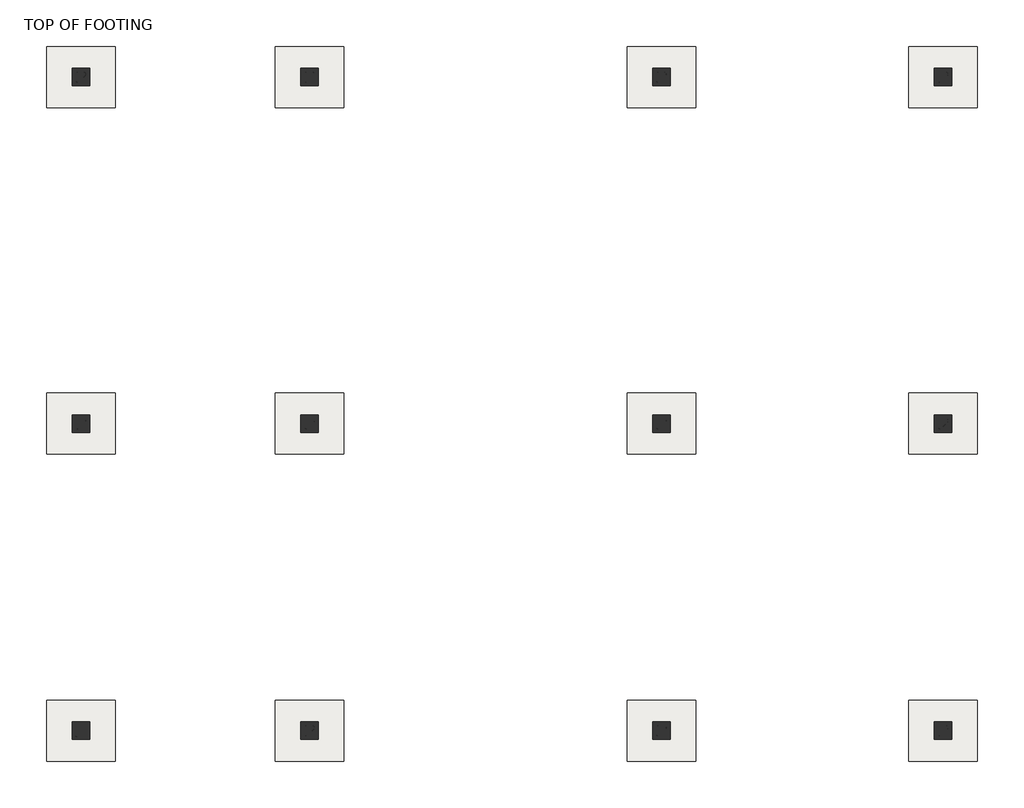
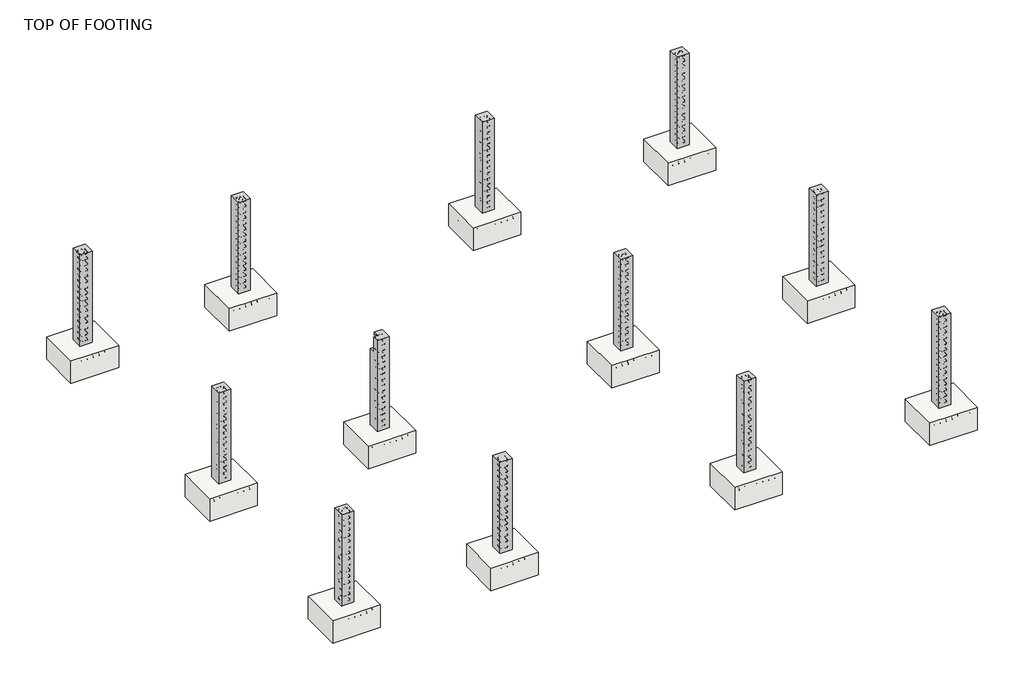
# One storey, part 1 of 6: 12 columns, 12 slabs.
"""IFC4 building model written with IfcOpenShell, lengths in millimetres."""

from ifc_helpers import new_model, si_unit, frame, origin, place, context, project, spatial, polyline, outline, extrude, faceted_brep, transform, mapped, element, save
from components import m_footing_rectangular_f0562f77

model = new_model("IFC4")

# Units and contexts
model_context = context("Model", 3, world=origin())
ifc_project = project(units=[si_unit("LENGTHUNIT", "METRE", prefix="MILLI")], contexts=[model_context])

# Site, building, storey
site = spatial("IfcSite", under=ifc_project)
building = spatial("IfcBuilding", under=site)
storey = spatial("IfcBuildingStorey", under=building, Name="TOP OF FOOTING", Elevation=-1828.8)

# Columns
placement = place(None, origin())
element("IfcColumn", 1, ObjectType="M_Concrete-Rectangular-Column : 9\" X 9\"", at=placement, inside=storey, context=model_context, shape_type="SweptSolid", body=[
    extrude(outline(polyline([(-14809.4556799, 4426.9016651), (-14809.4556799, 4198.3016651), (-15038.0556799, 4198.3016651), (-15038.0556799, 4426.9016651), (-14809.4556799, 4426.9016651)])), frame((0.0, 0.0, -1828.8), z_axis=(0.0, 0.0, 1.0), x_axis=(1.0, 0.0, 0.0)), (0.0, 0.0, 1.0), 1828.8),
])
element("IfcColumn", 2, ObjectType="M_Concrete-Rectangular-Column : 9\" X 9\"", at=placement, inside=storey, context=model_context, shape_type="Brep", body=[
    faceted_brep([(-11812.2556799, 4426.9016651, -1828.8), (-11812.2556799, 4198.3016651, -1828.8), (-12040.8556799, 4198.3016651, -1828.8), (-12040.8556799, 4426.9016651, -1828.8), (-11812.2556799, 4426.9016651, 0.0), (-11812.2556799, 4198.3016651, 0.0), (-11964.6556799, 4198.3016651, 0.0), (-12040.8556799, 4198.3016651, 0.0), (-12040.8556799, 4426.9016651, 0.0)], [[[0, 1, 2, 3]], [[4, 5, 1, 0]], [[5, 6, 7, 2, 1]], [[7, 8, 3, 2]], [[8, 4, 0, 3]], [[4, 8, 7, 6, 5]]]),
])
element("IfcColumn", 3, ObjectType="M_Concrete-Rectangular-Column : 9\" X 9\"", at=placement, inside=storey, context=model_context, shape_type="SweptSolid", body=[
    extrude(outline(polyline([(-7200.1673382, 4426.9016651), (-7200.1673382, 4198.3016651), (-7428.7673382, 4198.3016651), (-7428.7673382, 4426.9016651), (-7200.1673382, 4426.9016651)])), frame((0.0, 0.0, -1828.8), z_axis=(0.0, 0.0, 1.0), x_axis=(1.0, 0.0, 0.0)), (0.0, 0.0, 1.0), 1828.8),
])
element("IfcColumn", 4, ObjectType="M_Concrete-Rectangular-Column : 9\" X 9\"", at=placement, inside=storey, context=model_context, shape_type="SweptSolid", body=[
    extrude(outline(polyline([(-3506.4556799, 4426.9016651), (-3506.4556799, 4198.3016651), (-3735.0556799, 4198.3016651), (-3735.0556799, 4426.9016651), (-3506.4556799, 4426.9016651)])), frame((0.0, 0.0, -1828.8), z_axis=(0.0, 0.0, 1.0), x_axis=(1.0, 0.0, 0.0)), (0.0, 0.0, 1.0), 1828.8),
])
element("IfcColumn", 5, ObjectType="M_Concrete-Rectangular-Column : 9\" X 9\"", at=placement, inside=storey, context=model_context, shape_type="SweptSolid", body=[
    extrude(outline(polyline([(-3506.4556799, -118.4025279), (-3506.4556799, -347.0025279), (-3735.0556799, -347.0025279), (-3735.0556799, -118.4025279), (-3506.4556799, -118.4025279)])), frame((0.0, 0.0, -1828.8), z_axis=(0.0, 0.0, 1.0), x_axis=(1.0, 0.0, 0.0)), (0.0, 0.0, 1.0), 1828.8),
])
element("IfcColumn", 6, ObjectType="M_Concrete-Rectangular-Column : 9\" X 9\"", at=placement, inside=storey, context=model_context, shape_type="SweptSolid", body=[
    extrude(outline(polyline([(-7200.1673382, -118.4025279), (-7200.1673382, -347.0025279), (-7428.7673382, -347.0025279), (-7428.7673382, -118.4025279), (-7200.1673382, -118.4025279)])), frame((0.0, 0.0, -1828.8), z_axis=(0.0, 0.0, 1.0), x_axis=(1.0, 0.0, 0.0)), (0.0, 0.0, 1.0), 1828.8),
])
element("IfcColumn", 7, ObjectType="M_Concrete-Rectangular-Column : 9\" X 9\"", at=placement, inside=storey, context=model_context, shape_type="Brep", body=[
    faceted_brep([(-11812.2556799, -118.4025279, -1828.8), (-11812.2556799, -347.0025279, -1828.8), (-12040.8556799, -347.0025279, -1828.8), (-12040.8556799, -118.4025279, -1828.8), (-11812.2556799, -118.4025279, 0.0), (-11812.2556799, -347.0025279, 0.0), (-12040.8556799, -347.0025279, 0.0), (-12040.8556799, -232.7025279, 0.0), (-12040.8556799, -232.7025279, -300.0), (-12040.8556799, -118.4025279, -300.0), (-11964.6556799, -118.4025279, -300.0), (-11964.6556799, -118.4025279, 0.0), (-11964.6556799, -232.7025279, 0.0), (-11964.6556799, -232.7025279, -300.0)], [[[0, 1, 2, 3]], [[1, 0, 4, 5]], [[2, 1, 5, 6]], [[3, 2, 6, 7, 8, 9]], [[0, 3, 9, 10, 11, 4]], [[5, 4, 11, 12, 7, 6]], [[8, 13, 10, 9]], [[13, 12, 11, 10]], [[12, 13, 8, 7]]]),
])
element("IfcColumn", 8, ObjectType="M_Concrete-Rectangular-Column : 9\" X 9\"", at=placement, inside=storey, context=model_context, shape_type="Brep", body=[
    faceted_brep([(-14809.4556799, -118.4025279, -1828.8), (-14809.4556799, -347.0025279, -1828.8), (-15038.0556799, -347.0025279, -1828.8), (-15038.0556799, -118.4025279, -1828.8), (-14809.4556799, -118.4025279, 0.0), (-14809.4556799, -232.7025279, 0.0), (-14809.4556799, -347.0025279, 0.0), (-15038.0556799, -347.0025279, 0.0), (-15038.0556799, -118.4025279, 0.0)], [[[0, 1, 2, 3]], [[4, 5, 6, 1, 0]], [[6, 7, 2, 1]], [[7, 8, 3, 2]], [[8, 4, 0, 3]], [[4, 8, 7, 6, 5]]]),
])
element("IfcColumn", 9, ObjectType="M_Concrete-Rectangular-Column : 9\" X 9\"", at=placement, inside=storey, context=model_context, shape_type="SweptSolid", body=[
    extrude(outline(polyline([(-14809.4556799, -4145.5983349), (-14809.4556799, -4374.1983349), (-15038.0556799, -4374.1983349), (-15038.0556799, -4145.5983349), (-14809.4556799, -4145.5983349)])), frame((0.0, 0.0, -1828.8), z_axis=(0.0, 0.0, 1.0), x_axis=(1.0, 0.0, 0.0)), (0.0, 0.0, 1.0), 1828.8),
])
element("IfcColumn", 10, ObjectType="M_Concrete-Rectangular-Column : 9\" X 9\"", at=placement, inside=storey, context=model_context, shape_type="SweptSolid", body=[
    extrude(outline(polyline([(-11812.2556799, -4145.5983349), (-11812.2556799, -4374.1983349), (-12040.8556799, -4374.1983349), (-12040.8556799, -4145.5983349), (-11812.2556799, -4145.5983349)])), frame((0.0, 0.0, -1828.8), z_axis=(0.0, 0.0, 1.0), x_axis=(1.0, 0.0, 0.0)), (0.0, 0.0, 1.0), 1828.8),
])
element("IfcColumn", 11, ObjectType="M_Concrete-Rectangular-Column : 9\" X 9\"", at=placement, inside=storey, context=model_context, shape_type="SweptSolid", body=[
    extrude(outline(polyline([(-7200.1673382, -4145.5983349), (-7200.1673382, -4374.1983349), (-7428.7673382, -4374.1983349), (-7428.7673382, -4145.5983349), (-7200.1673382, -4145.5983349)])), frame((0.0, 0.0, -1828.8), z_axis=(0.0, 0.0, 1.0), x_axis=(1.0, 0.0, 0.0)), (0.0, 0.0, 1.0), 1828.8),
])
element("IfcColumn", 12, ObjectType="M_Concrete-Rectangular-Column : 9\" X 9\"", at=placement, inside=storey, context=model_context, shape_type="SweptSolid", body=[
    extrude(outline(polyline([(-3506.4556799, -4145.5983349), (-3506.4556799, -4374.1983349), (-3735.0556799, -4374.1983349), (-3735.0556799, -4145.5983349), (-3506.4556799, -4145.5983349)])), frame((0.0, 0.0, -1828.8), z_axis=(0.0, 0.0, 1.0), x_axis=(1.0, 0.0, 0.0)), (0.0, 0.0, 1.0), 1828.8),
])

# Slabs
element("IfcSlab", 13, ObjectType="M_Footing-Rectangular", at=placement, inside=storey, context=model_context, shape_type="SweptSolid", body=[
    extrude(outline(polyline([(-14473.7556799, 4712.6016651), (-14473.7556799, 3912.6016651), (-15373.7556799, 3912.6016651), (-15373.7556799, 4712.6016651), (-14473.7556799, 4712.6016651)])), frame((0.0, 0.0, -2278.8), z_axis=(0.0, 0.0, 1.0), x_axis=(1.0, 0.0, 0.0)), (0.0, 0.0, 1.0), 450.0),
])
element("IfcSlab", 14, ObjectType="M_Footing-Rectangular", at=placement, inside=storey, context=model_context, shape_type="SweptSolid", body=[
    extrude(outline(polyline([(-11476.5556799, 4712.6016651), (-11476.5556799, 3912.6016651), (-12376.5556799, 3912.6016651), (-12376.5556799, 4712.6016651), (-11476.5556799, 4712.6016651)])), frame((0.0, 0.0, -2278.8), z_axis=(0.0, 0.0, 1.0), x_axis=(1.0, 0.0, 0.0)), (0.0, 0.0, 1.0), 450.0),
])
element("IfcSlab", 15, ObjectType="M_Footing-Rectangular", at=placement, inside=storey, context=model_context, shape_type="SweptSolid", body=[
    extrude(outline(polyline([(-6864.4673382, 4712.6016651), (-6864.4673382, 3912.6016651), (-7764.4673382, 3912.6016651), (-7764.4673382, 4712.6016651), (-6864.4673382, 4712.6016651)])), frame((0.0, 0.0, -2278.8), z_axis=(0.0, 0.0, 1.0), x_axis=(1.0, 0.0, 0.0)), (0.0, 0.0, 1.0), 450.0),
])
element("IfcSlab", 16, ObjectType="M_Footing-Rectangular", at=placement, inside=storey, context=model_context, shape_type="SweptSolid", body=[
    extrude(outline(polyline([(-3170.7556799, 4712.6016651), (-3170.7556799, 3912.6016651), (-4070.7556799, 3912.6016651), (-4070.7556799, 4712.6016651), (-3170.7556799, 4712.6016651)])), frame((0.0, 0.0, -2278.8), z_axis=(0.0, 0.0, 1.0), x_axis=(1.0, 0.0, 0.0)), (0.0, 0.0, 1.0), 450.0),
])
element("IfcSlab", 17, ObjectType="M_Footing-Rectangular", at=placement, inside=storey, context=model_context, shape_type="SweptSolid", body=[
    extrude(outline(polyline([(-6864.4673382, 167.2974721), (-6864.4673382, -632.7025279), (-7764.4673382, -632.7025279), (-7764.4673382, 167.2974721), (-6864.4673382, 167.2974721)])), frame((0.0, 0.0, -2278.8), z_axis=(0.0, 0.0, 1.0), x_axis=(1.0, 0.0, 0.0)), (0.0, 0.0, 1.0), 450.0),
])
element("IfcSlab", 18, ObjectType="M_Footing-Rectangular", at=placement, inside=storey, context=model_context, shape_type="SweptSolid", body=[
    extrude(outline(polyline([(-3170.7556799, 167.2974721), (-3170.7556799, -632.7025279), (-4070.7556799, -632.7025279), (-4070.7556799, 167.2974721), (-3170.7556799, 167.2974721)])), frame((0.0, 0.0, -2278.8), z_axis=(0.0, 0.0, 1.0), x_axis=(1.0, 0.0, 0.0)), (0.0, 0.0, 1.0), 450.0),
])
m_footing_rectangular_shape = m_footing_rectangular_f0562f77(model_context)
element("IfcSlab", 19, ObjectType="M_Footing-Rectangular", at=placement, inside=storey, context=model_context, shape_type="MappedRepresentation", body=[
    mapped(m_footing_rectangular_shape, transform((-14923.7556799, -232.7025279, -1828.8), x_axis=(1.0, 0.0, 0.0), y_axis=(0.0, 1.0, 0.0), z_axis=(0.0, 0.0, 1.0))),
])
element("IfcSlab", 20, ObjectType="M_Footing-Rectangular", at=placement, inside=storey, context=model_context, shape_type="MappedRepresentation", body=[
    mapped(m_footing_rectangular_shape, transform((-11926.5556799, -232.7025279, -1828.8), x_axis=(1.0, 0.0, 0.0), y_axis=(0.0, 1.0, 0.0), z_axis=(0.0, 0.0, 1.0))),
])
element("IfcSlab", 21, ObjectType="M_Footing-Rectangular", at=placement, inside=storey, context=model_context, shape_type="MappedRepresentation", body=[
    mapped(m_footing_rectangular_shape, transform((-14923.7556799, -4259.8983349, -1828.8), x_axis=(1.0, 0.0, 0.0), y_axis=(0.0, 1.0, 0.0), z_axis=(0.0, 0.0, 1.0))),
])
element("IfcSlab", 22, ObjectType="M_Footing-Rectangular", at=placement, inside=storey, context=model_context, shape_type="MappedRepresentation", body=[
    mapped(m_footing_rectangular_shape, transform((-11926.5556799, -4259.8983349, -1828.8), x_axis=(1.0, 0.0, 0.0), y_axis=(0.0, 1.0, 0.0), z_axis=(0.0, 0.0, 1.0))),
])
element("IfcSlab", 23, ObjectType="M_Footing-Rectangular", at=placement, inside=storey, context=model_context, shape_type="MappedRepresentation", body=[
    mapped(m_footing_rectangular_shape, transform((-7314.4673382, -4259.8983349, -1828.8), x_axis=(1.0, 0.0, 0.0), y_axis=(0.0, 1.0, 0.0), z_axis=(0.0, 0.0, 1.0))),
])
element("IfcSlab", 24, ObjectType="M_Footing-Rectangular", at=placement, inside=storey, context=model_context, shape_type="MappedRepresentation", body=[
    mapped(m_footing_rectangular_shape, transform((-3620.7556799, -4259.8983349, -1828.8), x_axis=(1.0, 0.0, 0.0), y_axis=(0.0, 1.0, 0.0), z_axis=(0.0, 0.0, 1.0))),
])

save(model, "model.ifc")

# Revit data of these elements
# Grids (mm)
#   "A": line (-1541.632, 4312.602) -> (-20694.702, 4312.602)
#   "B": line (-1541.632, -232.703) -> (-20694.702, -232.703)
#   "C": line (-1541.632, -4259.898) -> (-20694.702, -4259.898)
# Type "M_Concrete-Rectangular-Column : 9\" X 9\""
#   b = 0' - 9"
#   h = 0' - 9"
#   Structural Material [instance default] = Concrete, Cast-in-Place gray
# Type "M_Footing-Rectangular"
#   Width = 2' - 11.43307"
#   Length = 2' - 7.49606"
#   Foundation Thickness = 1' - 5.71654"
#   Structural Material [instance default] = Concrete, Cast-in-Place gray
#   Assembly Code = ""
# Elements 1, 2, 3, 4, 5, 6, 7, 8, 9, 10, 11, 12 (IfcColumn, "M_Concrete-Rectangular-Column : 9\" X 9\"")
#   Structural Material = Concrete, Cast-in-Place gray
#   Phase Created = New Construction
#   Materials on its faces: "Concrete, Cast-in-Place gray"
# Elements 13, 14, 15, 16, 17, 18, 19, 20, 21, 22, 23, 24 (IfcSlab, "M_Footing-Rectangular")
#   Structural Material = Concrete, Cast-in-Place gray
#   Phase Created = New Construction
#   Materials on its faces: "Concrete, Cast-in-Place gray"
# Materials
#   "Concrete, Cast-in-Place gray": class "Concrete", colour RGB 192 192 192, transparency 0, Description = "Cast-in-place concrete", Cost = 0
